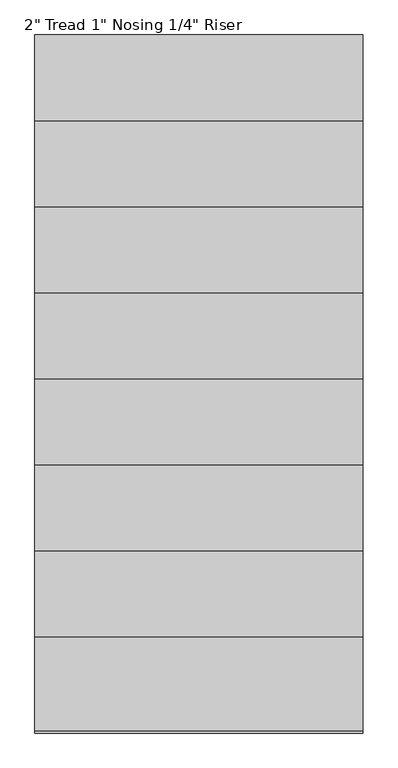
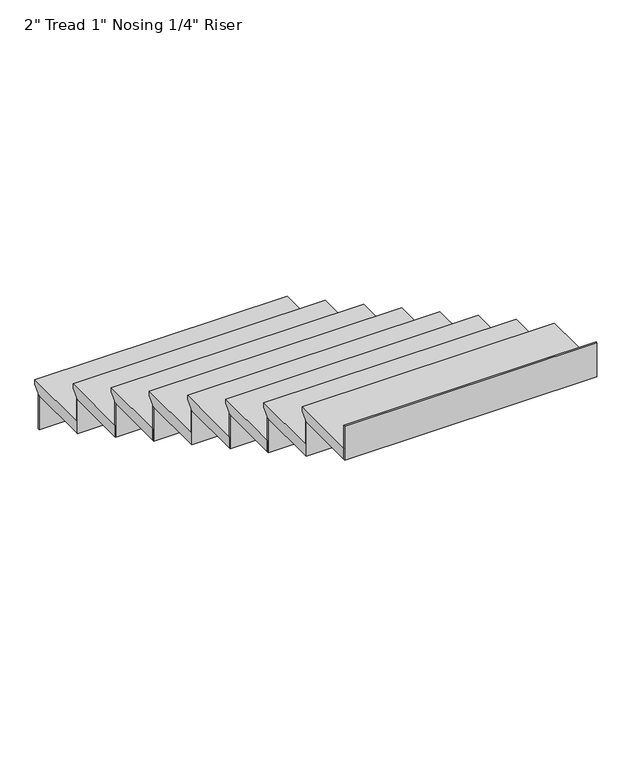
"""IFC4 building model written with IfcOpenShell, lengths in millimetres: stair flight geometry."""

from ifc_helpers import new_model, si_unit, frame, origin, place, context, project, spatial, polyline, outline, extrude, source, transform, mapped, element, save


def stair_flight_f2f674f0(model_context):
    return source(origin(), model_context, "Body", "SweptSolid", [
        extrude(outline(polyline([(-2204.7834702, 1828.8), (-1899.9834702, 1828.8), (-1899.9834702, 1809.75), (-1925.3834702, 1784.35), (-1925.3834702, 1778.0), (-2204.7834702, 1778.0), (-2204.7834702, 1828.8)])), frame((2385.53354, 0.0, 0.0), z_axis=(1.0, 0.0, 0.0), x_axis=(0.0, 1.0, 0.0)), (0.0, 0.0, 1.0), 1066.8),
        extrude(outline(polyline([(2385.53354, -1931.7334702), (2385.53354, -1925.3834702), (3452.33354, -1925.3834702), (3452.33354, -1931.7334702), (2385.53354, -1931.7334702)])), frame((0.0, 0.0, 1625.6), z_axis=(0.0, 0.0, 1.0), x_axis=(1.0, 0.0, 0.0)), (0.0, 0.0, 1.0), 152.4),
        extrude(outline(polyline([(2385.53354, -2211.1334702), (2385.53354, -2204.7834702), (3452.33354, -2204.7834702), (3452.33354, -2211.1334702), (2385.53354, -2211.1334702)])), frame((0.0, 0.0, 1778.0), z_axis=(0.0, 0.0, 1.0), x_axis=(1.0, 0.0, 0.0)), (0.0, 0.0, 1.0), 152.4),
        extrude(outline(polyline([(-2484.1834702, 1981.2), (-2179.3834702, 1981.2), (-2179.3834702, 1962.15), (-2204.7834702, 1936.75), (-2204.7834702, 1930.4), (-2484.1834702, 1930.4), (-2484.1834702, 1981.2)])), frame((2385.53354, 0.0, 0.0), z_axis=(1.0, 0.0, 0.0), x_axis=(0.0, 1.0, 0.0)), (0.0, 0.0, 1.0), 1066.8),
        extrude(outline(polyline([(2385.53354, -2490.5334702), (2385.53354, -2484.1834702), (3452.33354, -2484.1834702), (3452.33354, -2490.5334702), (2385.53354, -2490.5334702)])), frame((0.0, 0.0, 1930.4), z_axis=(0.0, 0.0, 1.0), x_axis=(1.0, 0.0, 0.0)), (0.0, 0.0, 1.0), 152.4),
        extrude(outline(polyline([(-2763.5834702, 2133.6), (-2458.7834702, 2133.6), (-2458.7834702, 2114.55), (-2484.1834702, 2089.15), (-2484.1834702, 2082.8), (-2763.5834702, 2082.8), (-2763.5834702, 2133.6)])), frame((2385.53354, 0.0, 0.0), z_axis=(1.0, 0.0, 0.0), x_axis=(0.0, 1.0, 0.0)), (0.0, 0.0, 1.0), 1066.8),
        extrude(outline(polyline([(2385.53354, -2769.9334702), (2385.53354, -2763.5834702), (3452.33354, -2763.5834702), (3452.33354, -2769.9334702), (2385.53354, -2769.9334702)])), frame((0.0, 0.0, 2082.8), z_axis=(0.0, 0.0, 1.0), x_axis=(1.0, 0.0, 0.0)), (0.0, 0.0, 1.0), 152.4),
        extrude(outline(polyline([(-3042.9834702, 2286.0), (-2738.1834702, 2286.0), (-2738.1834702, 2266.95), (-2763.5834702, 2241.55), (-2763.5834702, 2235.2), (-3042.9834702, 2235.2), (-3042.9834702, 2286.0)])), frame((2385.53354, 0.0, 0.0), z_axis=(1.0, 0.0, 0.0), x_axis=(0.0, 1.0, 0.0)), (0.0, 0.0, 1.0), 1066.8),
        extrude(outline(polyline([(2385.53354, -3049.3334702), (2385.53354, -3042.9834702), (3452.33354, -3042.9834702), (3452.33354, -3049.3334702), (2385.53354, -3049.3334702)])), frame((0.0, 0.0, 2235.2), z_axis=(0.0, 0.0, 1.0), x_axis=(1.0, 0.0, 0.0)), (0.0, 0.0, 1.0), 152.4),
        extrude(outline(polyline([(-3322.3834702, 2438.4), (-3017.5834702, 2438.4), (-3017.5834702, 2419.35), (-3042.9834702, 2393.95), (-3042.9834702, 2387.6), (-3322.3834702, 2387.6), (-3322.3834702, 2438.4)])), frame((2385.53354, 0.0, 0.0), z_axis=(1.0, 0.0, 0.0), x_axis=(0.0, 1.0, 0.0)), (0.0, 0.0, 1.0), 1066.8),
        extrude(outline(polyline([(2385.53354, -3328.7334702), (2385.53354, -3322.3834702), (3452.33354, -3322.3834702), (3452.33354, -3328.7334702), (2385.53354, -3328.7334702)])), frame((0.0, 0.0, 2387.6), z_axis=(0.0, 0.0, 1.0), x_axis=(1.0, 0.0, 0.0)), (0.0, 0.0, 1.0), 152.4),
        extrude(outline(polyline([(-3601.7834702, 2590.8), (-3296.9834702, 2590.8), (-3296.9834702, 2571.75), (-3322.3834702, 2546.35), (-3322.3834702, 2540.0), (-3601.7834702, 2540.0), (-3601.7834702, 2590.8)])), frame((2385.53354, 0.0, 0.0), z_axis=(1.0, 0.0, 0.0), x_axis=(0.0, 1.0, 0.0)), (0.0, 0.0, 1.0), 1066.8),
        extrude(outline(polyline([(2385.53354, -3608.1334702), (2385.53354, -3601.7834702), (3452.33354, -3601.7834702), (3452.33354, -3608.1334702), (2385.53354, -3608.1334702)])), frame((0.0, 0.0, 2540.0), z_axis=(0.0, 0.0, 1.0), x_axis=(1.0, 0.0, 0.0)), (0.0, 0.0, 1.0), 152.4),
        extrude(outline(polyline([(-3881.1834702, 2743.2), (-3576.3834702, 2743.2), (-3576.3834702, 2724.15), (-3601.7834702, 2698.75), (-3601.7834702, 2692.4), (-3881.1834702, 2692.4), (-3881.1834702, 2743.2)])), frame((2385.53354, 0.0, 0.0), z_axis=(1.0, 0.0, 0.0), x_axis=(0.0, 1.0, 0.0)), (0.0, 0.0, 1.0), 1066.8),
        extrude(outline(polyline([(2385.53354, -3887.5334702), (2385.53354, -3881.1834702), (3452.33354, -3881.1834702), (3452.33354, -3887.5334702), (2385.53354, -3887.5334702)])), frame((0.0, 0.0, 2692.4), z_axis=(0.0, 0.0, 1.0), x_axis=(1.0, 0.0, 0.0)), (0.0, 0.0, 1.0), 152.4),
        extrude(outline(polyline([(2385.53354, -4166.9334702), (2385.53354, -4160.5834702), (3452.33354, -4160.5834702), (3452.33354, -4166.9334702), (2385.53354, -4166.9334702)])), frame((0.0, 0.0, 2844.8), z_axis=(0.0, 0.0, 1.0), x_axis=(1.0, 0.0, 0.0)), (0.0, 0.0, 1.0), 152.4),
        extrude(outline(polyline([(-4160.5834702, 2895.6), (-3855.7834702, 2895.6), (-3855.7834702, 2876.55), (-3881.1834702, 2851.15), (-3881.1834702, 2844.8), (-4160.5834702, 2844.8), (-4160.5834702, 2895.6)])), frame((2385.53354, 0.0, 0.0), z_axis=(1.0, 0.0, 0.0), x_axis=(0.0, 1.0, 0.0)), (0.0, 0.0, 1.0), 1066.8),
    ])


if __name__ == "__main__":
    model = new_model("IFC4")
    model_context = context("Model", 3, world=origin())
    ifc_project = project(units=[si_unit("LENGTHUNIT", "METRE", prefix="MILLI")], contexts=[model_context])
    site = spatial("IfcSite", under=ifc_project)
    building = spatial("IfcBuilding", under=site)
    placement = place(None, origin())
    stair_flight_shape = stair_flight_f2f674f0(model_context)
    element("IfcStairFlight", 1, ObjectType="2\" Tread 1\" Nosing 1/4\" Riser", at=placement, inside=building, context=model_context, shape_type="MappedRepresentation", body=[
        mapped(stair_flight_shape, transform((0.0, 0.0, 0.0), x_axis=(1.0, 0.0, 0.0), y_axis=(0.0, 1.0, 0.0), z_axis=(0.0, 0.0, 1.0))),
    ])
    save(model, "model.ifc")
